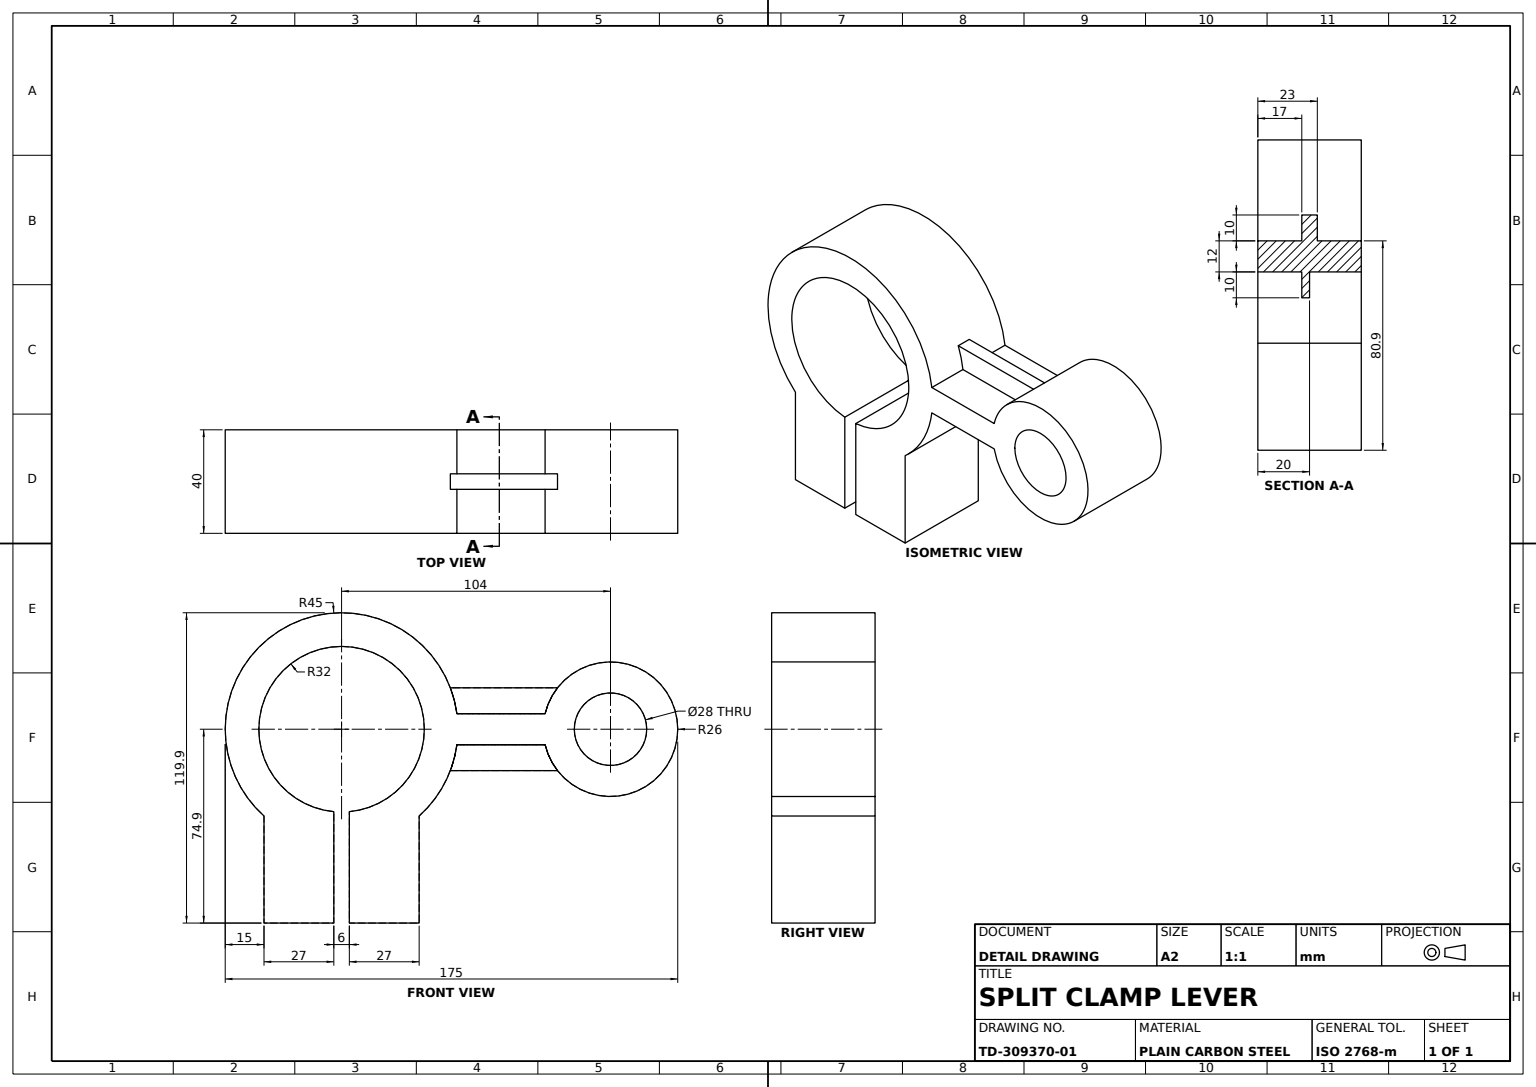
SolidWorks part; units mm, degrees
material "Plain Carbon Steel"
ref_plane "Front Plane" through (0, 0, 0) normal (0, 0, 1) x (1, 0, 0)
ref_plane "Top Plane" through (0, 0, 0) normal (0, 1, 0) x (1, 0, 0)
ref_plane "Right Plane" through (0, 0, 0) normal (1, 0, 0) x (0, 0, -1)
sketch "Clamp Body Sketch" plane through (0, 0, 0) normal (0, 0, 1) x (1, 0, 0)
  line L3 (52, -6) -> (78.7018, -6)
  line L4 (52, 6) -> (78.7018, 6)
  line L5 (52, 6) -> (44.5982, 6)
  line L7 (44.5982, -6) -> (52, -6)
  arc A1 (78.7018, -6) -> (78.7018, 6) centre (104, 0) ccw
  arc A4 (44.5982, 6) -> (44.5982, -6) centre (0, 0) ccw
  dimension "D1" = 90
  dimension "D2" = 52
  dimension "D3" = 26
  dimension "D4" = 45
  dimension "D5" = 25.2982
  dimension "D6" = 52
  dimension "D7" = 59.4018
extrude "Clamp Body" add sketch "Clamp Body Sketch" along normal blind 40
sketch "Pin Bore Sketch" plane through (0, 0, 40) normal (0, 0, 1) x (1, 0, 0)
  circle A0 centre (104, 0) radius 14
  dimension "D1" = 28
  dimension "D2" = 28
extrude "Pin Bore Ø28" cut sketch "Pin Bore Sketch" against normal blind 40
sketch "Clamp Bore and Slit Sketch" plane through (0, 0, 40) normal (0, 0, 1) x (1, 0, 0)
  line L0 (78.7018, 6) -> (44.5982, 6) construction
  line L2 (3, -76) -> (3, -31.8591)
  line L4 (-3, -31.8591) -> (-3, -76)
  line L6 (3, -76) -> (30, -76)
  line L7 (30, -76) -> (30, -11.1355)
  line L8 (-3, -76) -> (-30, -76)
  line L9 (-30, -76) -> (-30, -11.1355)
  arc A0 (3, -31.8591) -> (-3, -31.8591) centre (0, 0) ccw
  arc M4 (44.5982, 6) -> (44.5982, -6) centre (0, 0) ccw
  dimension "D1" = 64
  dimension "D2" = 32
  dimension "D3" = 14.5982
  dimension "D4" = 41.5982
  dimension "D5" = 82
extrude "Clamp Bore Ø64 and Slit" cut sketch "Clamp Bore and Slit Sketch" against normal blind 40 contours A0 L4 L2 M4
sketch "Lever Arm Sketch" plane through (0, 0, 40) normal (0, 0, 1) x (1, 0, 0)
  line L0 (-3, -44.8999) -> (-3, -74.8999)
  line L1 (-3, -74.8999) -> (-30, -74.8999)
  line L2 (-30, -74.8999) -> (-30, -33.541)
  line L3 (3, -44.8999) -> (3, -74.8999)
  line L4 (3, -74.8999) -> (30, -74.8999)
  line L5 (30, -74.8999) -> (30, -33.541)
  line L6 (3, -44.8999) -> (3, -31.8591) construction
  line L7 (78.7018, 6) -> (44.5982, 6) construction
  arc A0 (-30, -33.541) -> (-3, -44.8999) centre (0, 0) ccw
  arc A1 (3, -44.8999) -> (30, -33.541) centre (0, 0) ccw
  dimension "D1" = 90
  dimension "D2" = 27
  dimension "D3" = 80.8999
extrude "Lever Arm" add sketch "Lever Arm Sketch" against normal blind 40
sketch "Arm Web A Sketch" plane through (0, 6, 0) normal (0, 1, 0) x (1, 0, 0)
  line L0 (44.5982, -40) -> (44.5982, 0) construction
  line L1 (78.7018, 0) -> (44.5982, 0) construction
  line L2 (32.9126, -20) -> (32.9126, -17)
  line L3 (32.9126, -17) -> (88.9472, -17)
  line L4 (88.9472, -17) -> (88.9472, -23)
  line L5 (88.9472, -23) -> (32.9126, -23)
  line L6 (32.9126, -23) -> (32.9126, -20)
  dimension "D1" = 44.349
  dimension "D2" = 11.6856
  dimension "D3" = 17
  dimension "D4" = 20
extrude "Arm Web A" add sketch "Arm Web A Sketch" along normal blind 10
sketch "Arm Web B Sketch" plane through (0, -6, 0) normal (0, -1, 0) x (1, 0, 0)
  line L0 (78.7018, 40) -> (78.7018, 0) construction
  line L1 (44.5982, 40) -> (44.5982, 0) construction
  line L2 (44.5982, 23) -> (37.4933, 23)
  line L3 (37.4933, 23) -> (37.4933, 20)
  line L4 (37.4933, 20) -> (86.3405, 20)
  line L5 (86.3405, 20) -> (86.3405, 23)
  line L6 (86.3405, 23) -> (44.5982, 23)
  line L7 (44.5982, 0) -> (78.7018, 0) construction
  dimension "D1" = 7.6387
  dimension "D2" = 41.2084
  dimension "D3" = 20
  dimension "D4" = 23
extrude "Arm Web B" add sketch "Arm Web B Sketch" along normal blind 10
